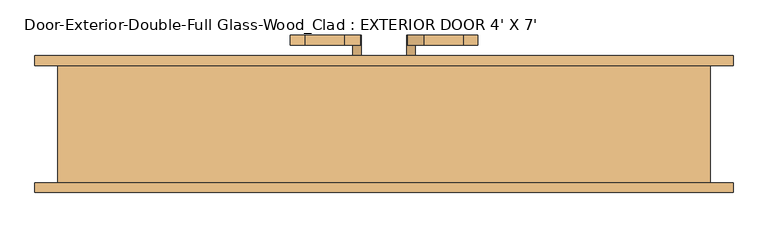
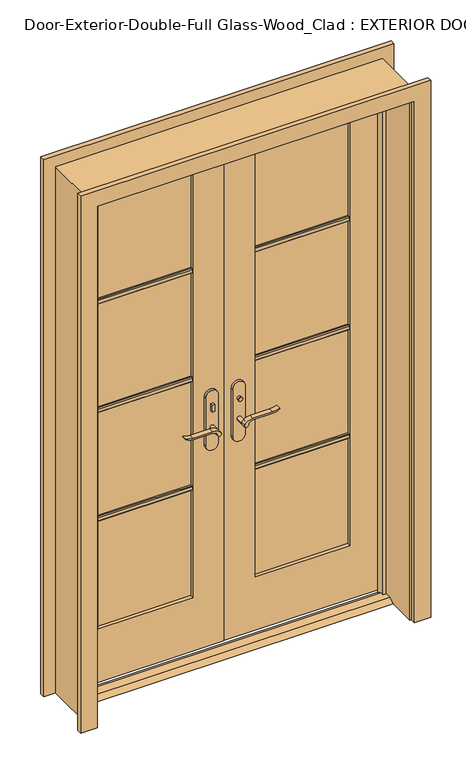
"""IFC4 building model written with IfcOpenShell, lengths in millimetres: door geometry, Door-Exterior-Double-Full Glass-Wood_Clad : EXTERIOR DOOR 4' X 7'."""

from ifc_helpers import new_model, si_unit, point, frame, frame_2d, origin, place, context, project, spatial, polyline, circle_curve, trimmed, segment, composite_curve, outline, extrude, faceted_brep, source, transform, mapped, element, save


def door_exterior_double_full_glass_wood_clad_exterior_door_4_x_3788f36b(model_context):
    return source(origin(), model_context, "Body", "SolidModel", [
        extrude(outline(polyline([(19.05, 12.7), (53.975, 12.7), (79.375, 0.0), (-6.35, 0.0), (19.05, 12.7)])), frame((-609.6, 0.0, 0.0), z_axis=(1.0, 0.0, 0.0), x_axis=(0.0, 1.0, 0.0)), (0.0, 0.0, 1.0), 1219.2),
        extrude(outline(polyline([(-47.4019111, 56.2), (-57.4019111, 56.2), (-57.4019111, 66.2), (-47.4019111, 66.2), (-47.4019111, 56.2)])), frame((0.0, 0.0, 981.9), z_axis=(0.0, 0.0, 1.0), x_axis=(1.0, 0.0, 0.0)), (0.0, 0.0, 1.0), 30.0),
        extrude(outline(composite_curve([segment(trimmed(circle_curve(frame_2d((996.9, -52.4019111)), 8.0), [point((996.9, -60.4019111))], [point((996.9, -44.4019111))], False, "CARTESIAN"), True, "CONTINUOUS"), segment(trimmed(circle_curve(frame_2d((996.9, -52.4019111)), 8.0), [point((996.9, -44.4019111))], [point((996.9, -60.4019111))], False, "CARTESIAN"), True, "CONTINUOUS")], self_intersect=False)), frame((0.0, 121.125, 0.0), z_axis=(0.0, 1.0, 0.0), x_axis=(0.0, 0.0, 1.0)), (0.0, 0.0, 1.0), 10.0),
        extrude(outline(composite_curve([segment(trimmed(circle_curve(frame_2d((897.1555521, -76.0694241)), 37.2832219), [point((919.0523287, -45.8937749))], [point((934.4, -77.7693445))], False, "CARTESIAN"), True, "CONTINUOUS"), segment(polyline([(934.4, -77.7693445), (934.4, -154.045502)]), True, "CONTINUOUS"), segment(trimmed(circle_curve(frame_2d((1017.6850638, -153.9791202)), 83.2850902), [point((934.4, -154.045502))], [point((939.4, -182.4019111))], True, "CARTESIAN"), True, "CONTINUOUS"), segment(polyline([(939.4, -182.4019111), (936.6135558, -182.4019111)]), True, "CONTINUOUS"), segment(trimmed(circle_curve(frame_2d((986.6709207, -150.4622499)), 59.3791355), [point((936.6135558, -182.4019111))], [point((927.4, -154.045502))], False, "CARTESIAN"), True, "CONTINUOUS"), segment(polyline([(927.4, -154.045502), (927.4, -77.7881013)]), True, "CONTINUOUS"), segment(trimmed(circle_curve(frame_2d((909.2738613, -77.7881013)), 18.1261387), [point((927.4, -77.7881013))], [point((914.4, -60.4019111))], True, "CARTESIAN"), True, "CONTINUOUS"), segment(trimmed(circle_curve(frame_2d((914.4, -52.4019111)), 8.0), [point((914.4, -60.4019111))], [point((919.0523287, -45.8937749))], False, "CARTESIAN"), True, "CONTINUOUS")], self_intersect=False)), frame((0.0, 16.2, 0.0), z_axis=(0.0, 1.0, 0.0), x_axis=(0.0, 0.0, 1.0)), (0.0, 0.0, 1.0), 20.0),
        extrude(outline(composite_curve([segment(trimmed(circle_curve(frame_2d((914.4, -52.4019111)), 8.0), [point((914.3999903, -60.4019111))], [point((919.0523287, -45.8937749))], False, "CARTESIAN"), True, "CONTINUOUS"), segment(trimmed(circle_curve(frame_2d((897.1555521, -76.0694241)), 37.2832219), [point((919.0523287, -45.8937749))], [point((934.4, -77.7693445))], False, "CARTESIAN"), True, "CONTINUOUS"), segment(polyline([(934.4, -77.7693445), (934.4, -154.045502)]), True, "CONTINUOUS"), segment(trimmed(circle_curve(frame_2d((1017.6850638, -153.9791202)), 83.2850902), [point((934.4, -154.045502))], [point((939.4, -182.4019111))], True, "CARTESIAN"), True, "CONTINUOUS"), segment(polyline([(939.4, -182.4019111), (936.6135558, -182.4019111)]), True, "CONTINUOUS"), segment(trimmed(circle_curve(frame_2d((986.6709207, -150.4622499)), 59.3791355), [point((936.6135558, -182.4019111))], [point((927.4, -154.045502))], False, "CARTESIAN"), True, "CONTINUOUS"), segment(polyline([(927.4, -154.045502), (927.4, -77.788099)]), True, "CONTINUOUS"), segment(trimmed(circle_curve(frame_2d((909.2738682, -77.788099)), 18.1261318), [point((927.4, -77.788099))], [point((914.3999903, -60.4019111))], True, "CARTESIAN"), True, "CONTINUOUS")], self_intersect=False)), frame((0.0, 151.125, 0.0), z_axis=(0.0, 1.0, 0.0), x_axis=(0.0, 0.0, 1.0)), (0.0, 0.0, 1.0), 20.0),
        extrude(outline(composite_curve([segment(trimmed(circle_curve(frame_2d((914.4, -52.4019111)), 8.0), [point((914.4, -60.4019111))], [point((914.4, -44.4019111))], False, "CARTESIAN"), True, "CONTINUOUS"), segment(trimmed(circle_curve(frame_2d((914.4, -52.4019111)), 8.0), [point((914.4, -44.4019111))], [point((914.4, -60.4019111))], False, "CARTESIAN"), True, "CONTINUOUS")], self_intersect=False)), frame((0.0, 36.2, 0.0), z_axis=(0.0, 1.0, 0.0), x_axis=(0.0, 0.0, 1.0)), (0.0, 0.0, 1.0), 30.0),
        extrude(outline(composite_curve([segment(trimmed(circle_curve(frame_2d((914.4, -52.4019111)), 8.0), [point((914.4, -60.4019111))], [point((914.4, -44.4019111))], False, "CARTESIAN"), True, "CONTINUOUS"), segment(trimmed(circle_curve(frame_2d((914.4, -52.4019111)), 8.0), [point((914.4, -44.4019111))], [point((914.4, -60.4019111))], False, "CARTESIAN"), True, "CONTINUOUS")], self_intersect=False)), frame((0.0, 121.125, 0.0), z_axis=(0.0, 1.0, 0.0), x_axis=(0.0, 0.0, 1.0)), (0.0, 0.0, 1.0), 30.0),
        extrude(outline(composite_curve([segment(polyline([(844.4, -27.4019111), (1039.4, -27.4019111)]), True, "CONTINUOUS"), segment(trimmed(circle_curve(frame_2d((1039.4, -52.4019111)), 25.0), [point((1039.4, -27.4019111))], [point((1039.4, -77.4019111))], False, "CARTESIAN"), True, "CONTINUOUS"), segment(polyline([(1039.4, -77.4019111), (844.4, -77.4019111)]), True, "CONTINUOUS"), segment(trimmed(circle_curve(frame_2d((844.4, -52.4019111)), 25.0), [point((844.4, -77.4019111))], [point((844.4, -27.4019111))], False, "CARTESIAN"), True, "CONTINUOUS")], self_intersect=False)), frame((0.0, 66.2, 0.0), z_axis=(0.0, 1.0, 0.0), x_axis=(0.0, 0.0, 1.0)), (0.0, 0.0, 1.0), 10.0),
        extrude(outline(composite_curve([segment(polyline([(844.4, -27.4019111), (1039.4, -27.4019111)]), True, "CONTINUOUS"), segment(trimmed(circle_curve(frame_2d((1039.4, -52.4019111)), 25.0), [point((1039.4, -27.4019111))], [point((1039.4, -77.4019111))], False, "CARTESIAN"), True, "CONTINUOUS"), segment(polyline([(1039.4, -77.4019111), (844.4, -77.4019111)]), True, "CONTINUOUS"), segment(trimmed(circle_curve(frame_2d((844.4, -52.4019111)), 25.0), [point((844.4, -77.4019111))], [point((844.4, -27.4019111))], False, "CARTESIAN"), True, "CONTINUOUS")], self_intersect=False)), frame((0.0, 111.125, 0.0), z_axis=(0.0, 1.0, 0.0), x_axis=(0.0, 0.0, 1.0)), (0.0, 0.0, 1.0), 10.0),
        extrude(outline(polyline([(47.3875, 131.125), (57.3875, 131.125), (57.3875, 121.125), (47.3875, 121.125), (47.3875, 131.125)])), frame((0.0, 0.0, 981.9), z_axis=(0.0, 0.0, 1.0), x_axis=(1.0, 0.0, 0.0)), (0.0, 0.0, 1.0), 30.0),
        extrude(outline(composite_curve([segment(trimmed(circle_curve(frame_2d((996.9, 52.3875)), 8.0), [point((996.9, 60.3875))], [point((996.9, 44.3875))], False, "CARTESIAN"), True, "CONTINUOUS"), segment(trimmed(circle_curve(frame_2d((996.9, 52.3875)), 8.0), [point((996.9, 44.3875))], [point((996.9, 60.3875))], False, "CARTESIAN"), True, "CONTINUOUS")], self_intersect=False)), frame((0.0, 56.2, 0.0), z_axis=(0.0, 1.0, 0.0), x_axis=(0.0, 0.0, 1.0)), (0.0, 0.0, 1.0), 10.0),
        extrude(outline(composite_curve([segment(trimmed(circle_curve(frame_2d((914.4, 52.3875)), 8.0), [point((919.0523287, 45.8793637))], [point((914.4, 60.3875))], False, "CARTESIAN"), True, "CONTINUOUS"), segment(trimmed(circle_curve(frame_2d((909.2738613, 77.7736901)), 18.1261387), [point((914.4, 60.3875))], [point((927.4, 77.7736901))], True, "CARTESIAN"), True, "CONTINUOUS"), segment(polyline([(927.4, 77.7736901), (927.4, 154.0310909)]), True, "CONTINUOUS"), segment(trimmed(circle_curve(frame_2d((986.6709207, 150.4478388)), 59.3791355), [point((927.4, 154.0310909))], [point((936.6135558, 182.3875))], False, "CARTESIAN"), True, "CONTINUOUS"), segment(polyline([(936.6135558, 182.3875), (939.4, 182.3875)]), True, "CONTINUOUS"), segment(trimmed(circle_curve(frame_2d((1017.6850638, 153.9647091)), 83.2850902), [point((939.4, 182.3875))], [point((934.4, 154.0310909))], True, "CARTESIAN"), True, "CONTINUOUS"), segment(polyline([(934.4, 154.0310909), (934.4, 77.7549333)]), True, "CONTINUOUS"), segment(trimmed(circle_curve(frame_2d((897.1555521, 76.0550129)), 37.2832219), [point((934.4, 77.7549333))], [point((919.0523287, 45.8793637))], False, "CARTESIAN"), True, "CONTINUOUS")], self_intersect=False)), frame((0.0, 151.125, 0.0), z_axis=(0.0, 1.0, 0.0), x_axis=(0.0, 0.0, 1.0)), (0.0, 0.0, 1.0), 20.0),
        extrude(outline(composite_curve([segment(trimmed(circle_curve(frame_2d((909.2738682, 77.7736878)), 18.1261318), [point((914.3999903, 60.3875))], [point((927.4, 77.7736878))], True, "CARTESIAN"), True, "CONTINUOUS"), segment(polyline([(927.4, 77.7736878), (927.4, 154.0310909)]), True, "CONTINUOUS"), segment(trimmed(circle_curve(frame_2d((986.6709207, 150.4478388)), 59.3791355), [point((927.4, 154.0310909))], [point((936.6135558, 182.3875))], False, "CARTESIAN"), True, "CONTINUOUS"), segment(polyline([(936.6135558, 182.3875), (939.4, 182.3875)]), True, "CONTINUOUS"), segment(trimmed(circle_curve(frame_2d((1017.6850638, 153.9647091)), 83.2850902), [point((939.4, 182.3875))], [point((934.4, 154.0310909))], True, "CARTESIAN"), True, "CONTINUOUS"), segment(polyline([(934.4, 154.0310909), (934.4, 77.7549333)]), True, "CONTINUOUS"), segment(trimmed(circle_curve(frame_2d((897.1555521, 76.0550129)), 37.2832219), [point((934.4, 77.7549333))], [point((919.0523287, 45.8793637))], False, "CARTESIAN"), True, "CONTINUOUS"), segment(trimmed(circle_curve(frame_2d((914.4, 52.3875)), 8.0), [point((919.0523287, 45.8793637))], [point((914.3999903, 60.3875))], False, "CARTESIAN"), True, "CONTINUOUS")], self_intersect=False)), frame((0.0, 16.2, 0.0), z_axis=(0.0, 1.0, 0.0), x_axis=(0.0, 0.0, 1.0)), (0.0, 0.0, 1.0), 20.0),
        extrude(outline(composite_curve([segment(trimmed(circle_curve(frame_2d((914.4, 52.3875)), 8.0), [point((914.4, 60.3875))], [point((914.4, 44.3875))], False, "CARTESIAN"), True, "CONTINUOUS"), segment(trimmed(circle_curve(frame_2d((914.4, 52.3875)), 8.0), [point((914.4, 44.3875))], [point((914.4, 60.3875))], False, "CARTESIAN"), True, "CONTINUOUS")], self_intersect=False)), frame((0.0, 121.125, 0.0), z_axis=(0.0, 1.0, 0.0), x_axis=(0.0, 0.0, 1.0)), (0.0, 0.0, 1.0), 30.0),
        extrude(outline(composite_curve([segment(trimmed(circle_curve(frame_2d((914.4, 52.3875)), 8.0), [point((914.4, 60.3875))], [point((914.4, 44.3875))], False, "CARTESIAN"), True, "CONTINUOUS"), segment(trimmed(circle_curve(frame_2d((914.4, 52.3875)), 8.0), [point((914.4, 44.3875))], [point((914.4, 60.3875))], False, "CARTESIAN"), True, "CONTINUOUS")], self_intersect=False)), frame((0.0, 36.2, 0.0), z_axis=(0.0, 1.0, 0.0), x_axis=(0.0, 0.0, 1.0)), (0.0, 0.0, 1.0), 30.0),
        extrude(outline(composite_curve([segment(trimmed(circle_curve(frame_2d((844.4, 52.3875)), 25.0), [point((844.4, 27.3875))], [point((844.4, 77.3875))], False, "CARTESIAN"), True, "CONTINUOUS"), segment(polyline([(844.4, 77.3875), (1039.4, 77.3875)]), True, "CONTINUOUS"), segment(trimmed(circle_curve(frame_2d((1039.4, 52.3875)), 25.0), [point((1039.4, 77.3875))], [point((1039.4, 27.3875))], False, "CARTESIAN"), True, "CONTINUOUS"), segment(polyline([(1039.4, 27.3875), (844.4, 27.3875)]), True, "CONTINUOUS")], self_intersect=False)), frame((0.0, 111.125, 0.0), z_axis=(0.0, 1.0, 0.0), x_axis=(0.0, 0.0, 1.0)), (0.0, 0.0, 1.0), 10.0),
        extrude(outline(composite_curve([segment(trimmed(circle_curve(frame_2d((844.4, 52.3875)), 25.0), [point((844.4, 27.3875))], [point((844.4, 77.3875))], False, "CARTESIAN"), True, "CONTINUOUS"), segment(polyline([(844.4, 77.3875), (1039.4, 77.3875)]), True, "CONTINUOUS"), segment(trimmed(circle_curve(frame_2d((1039.4, 52.3875)), 25.0), [point((1039.4, 77.3875))], [point((1039.4, 27.3875))], False, "CARTESIAN"), True, "CONTINUOUS"), segment(polyline([(1039.4, 27.3875), (844.4, 27.3875)]), True, "CONTINUOUS")], self_intersect=False)), frame((0.0, 66.2, 0.0), z_axis=(0.0, 1.0, 0.0), x_axis=(0.0, 0.0, 1.0)), (0.0, 0.0, 1.0), 10.0),
        extrude(outline(polyline([(90.17, 1578.371875), (90.17, 1559.321875), (83.82, 1559.321875), (80.645, 1562.496875), (80.645, 1575.196875), (83.82, 1578.371875), (90.17, 1578.371875)])), frame((120.65, 0.0, 0.0), z_axis=(1.0, 0.0, 0.0), x_axis=(0.0, 1.0, 0.0)), (0.0, 0.0, 1.0), 368.3),
        extrude(outline(polyline([(90.17, 1132.68125), (90.17, 1113.63125), (83.82, 1113.63125), (80.645, 1116.80625), (80.645, 1129.50625), (83.82, 1132.68125), (90.17, 1132.68125)])), frame((120.65, 0.0, 0.0), z_axis=(1.0, 0.0, 0.0), x_axis=(0.0, 1.0, 0.0)), (0.0, 0.0, 1.0), 368.3),
        extrude(outline(polyline([(90.17, 686.990625), (90.17, 667.940625), (83.82, 667.940625), (80.645, 671.115625), (80.645, 683.815625), (83.82, 686.990625), (90.17, 686.990625)])), frame((120.65, 0.0, 0.0), z_axis=(1.0, 0.0, 0.0), x_axis=(0.0, 1.0, 0.0)), (0.0, 0.0, 1.0), 368.3),
        extrude(outline(polyline([(97.155, 1578.371875), (103.505, 1578.371875), (106.68, 1575.196875), (106.68, 1562.496875), (103.505, 1559.321875), (97.155, 1559.321875), (97.155, 1578.371875)])), frame((-488.95, 0.0, 0.0), z_axis=(1.0, 0.0, 0.0), x_axis=(0.0, 1.0, 0.0)), (0.0, 0.0, 1.0), 368.3),
        extrude(outline(polyline([(97.155, 1132.68125), (103.505, 1132.68125), (106.68, 1129.50625), (106.68, 1116.80625), (103.505, 1113.63125), (97.155, 1113.63125), (97.155, 1132.68125)])), frame((-488.95, 0.0, 0.0), z_axis=(1.0, 0.0, 0.0), x_axis=(0.0, 1.0, 0.0)), (0.0, 0.0, 1.0), 368.3),
        extrude(outline(polyline([(97.155, 686.990625), (103.505, 686.990625), (106.68, 683.815625), (106.68, 671.115625), (103.505, 667.940625), (97.155, 667.940625), (97.155, 686.990625)])), frame((-488.95, 0.0, 0.0), z_axis=(1.0, 0.0, 0.0), x_axis=(0.0, 1.0, 0.0)), (0.0, 0.0, 1.0), 368.3),
        extrude(outline(polyline([(97.155, 1578.371875), (103.505, 1578.371875), (106.68, 1575.196875), (106.68, 1562.496875), (103.505, 1559.321875), (97.155, 1559.321875), (97.155, 1578.371875)])), frame((120.65, 0.0, 0.0), z_axis=(1.0, 0.0, 0.0), x_axis=(0.0, 1.0, 0.0)), (0.0, 0.0, 1.0), 368.3),
        extrude(outline(polyline([(97.155, 1132.68125), (103.505, 1132.68125), (106.68, 1129.50625), (106.68, 1116.80625), (103.505, 1113.63125), (97.155, 1113.63125), (97.155, 1132.68125)])), frame((120.65, 0.0, 0.0), z_axis=(1.0, 0.0, 0.0), x_axis=(0.0, 1.0, 0.0)), (0.0, 0.0, 1.0), 368.3),
        extrude(outline(polyline([(97.155, 686.990625), (103.505, 686.990625), (106.68, 683.815625), (106.68, 671.115625), (103.505, 667.940625), (97.155, 667.940625), (97.155, 686.990625)])), frame((120.65, 0.0, 0.0), z_axis=(1.0, 0.0, 0.0), x_axis=(0.0, 1.0, 0.0)), (0.0, 0.0, 1.0), 368.3),
        extrude(outline(polyline([(90.17, 1578.371875), (90.17, 1559.321875), (83.82, 1559.321875), (80.645, 1562.496875), (80.645, 1575.196875), (83.82, 1578.371875), (90.17, 1578.371875)])), frame((-488.95, 0.0, 0.0), z_axis=(1.0, 0.0, 0.0), x_axis=(0.0, 1.0, 0.0)), (0.0, 0.0, 1.0), 368.3),
        extrude(outline(polyline([(90.17, 1132.68125), (90.17, 1113.63125), (83.82, 1113.63125), (80.645, 1116.80625), (80.645, 1129.50625), (83.82, 1132.68125), (90.17, 1132.68125)])), frame((-488.95, 0.0, 0.0), z_axis=(1.0, 0.0, 0.0), x_axis=(0.0, 1.0, 0.0)), (0.0, 0.0, 1.0), 368.3),
        extrude(outline(polyline([(90.17, 686.990625), (90.17, 667.940625), (83.82, 667.940625), (80.645, 671.115625), (80.645, 683.815625), (83.82, 686.990625), (90.17, 686.990625)])), frame((-488.95, 0.0, 0.0), z_axis=(1.0, 0.0, 0.0), x_axis=(0.0, 1.0, 0.0)), (0.0, 0.0, 1.0), 368.3),
        extrude(outline(polyline([(0.0, 615.95), (0.0, 679.45), (2203.45, 679.45), (2203.45, -679.45), (0.0, -679.45), (0.0, -615.95), (2139.95, -615.95), (2139.95, 615.95), (0.0, 615.95)])), frame((0.0, -136.525, 0.0), z_axis=(0.0, 1.0, 0.0), x_axis=(0.0, 0.0, 1.0)), (0.0, 0.0, 1.0), 19.05),
        extrude(outline(polyline([(0.0, 615.95), (0.0, 679.45), (2203.45, 679.45), (2203.45, -679.45), (0.0, -679.45), (0.0, -615.95), (2139.95, -615.95), (2139.95, 615.95), (0.0, 615.95)])), frame((0.0, 111.125, 0.0), z_axis=(0.0, 1.0, 0.0), x_axis=(0.0, 0.0, 1.0)), (0.0, 0.0, 1.0), 19.05),
        faceted_brep([(635.0, 111.125, 0.0), (635.0, -117.475, 0.0), (609.6, -117.475, 0.0), (609.6, 41.275, 0.0), (596.9, 41.275, 0.0), (596.9, 76.2, 0.0), (609.6, 76.2, 0.0), (609.6, 111.125, 0.0), (635.0, 111.125, 2159.0), (635.0, -117.475, 2159.0), (-635.0, -117.475, 2159.0), (-635.0, -117.475, 0.0), (-609.6, -117.475, 0.0), (-609.6, -117.475, 2133.6), (609.6, -117.475, 2133.6), (609.6, 41.275, 2133.6), (-609.6, 41.275, 2133.6), (-609.6, 41.275, 0.0), (-596.9, 41.275, 0.0), (-596.9, 41.275, 2120.9), (596.9, 41.275, 2120.9), (596.9, 76.2, 2120.9), (1.5875, 76.2, 2120.9), (-1.6019111, 76.2, 2120.9), (-596.9, 76.2, 2120.9), (-596.9, 76.2, 0.0), (-609.6, 76.2, 0.0), (-609.6, 76.2, 2133.6), (-1.6019111, 76.2, 2133.6), (1.5875, 76.2, 2133.6), (609.6, 76.2, 2133.6), (609.6, 111.125, 2133.6), (1.5875, 111.125, 2133.6), (-1.6019111, 111.125, 2133.6), (-609.6, 111.125, 2133.6), (-609.6, 111.125, 0.0), (-635.0, 111.125, 0.0), (-635.0, 111.125, 2159.0)], [[[0, 1, 2, 3, 4, 5, 6, 7]], [[1, 0, 8, 9]], [[2, 1, 9, 10, 11, 12, 13, 14]], [[3, 2, 14, 15]], [[4, 3, 15, 16, 17, 18, 19, 20]], [[5, 4, 20, 21]], [[6, 5, 21, 22, 23, 24, 25, 26, 27, 28, 29, 30]], [[7, 6, 30, 31]], [[0, 7, 31, 32, 33, 34, 35, 36, 37, 8]], [[9, 8, 37, 10]], [[14, 13, 16, 15]], [[20, 19, 24, 23, 22, 21]], [[31, 30, 29, 28, 27, 34, 33, 32]], [[12, 11, 36, 35, 26, 25, 18, 17]], [[11, 10, 37, 36]], [[13, 12, 17, 16]], [[19, 18, 25, 24]], [[27, 26, 35, 34]]]),
        extrude(outline(polyline([(12.7, 609.6), (2133.6, 609.6), (2133.6, 1.5875), (12.7, 1.5875), (12.7, 609.6)]), holes=[polyline([(2014.5375, 120.65), (2014.5375, 488.95), (231.775, 488.95), (231.775, 120.65), (2014.5375, 120.65)])]), frame((0.0, 76.2, 0.0), z_axis=(0.0, 1.0, 0.0), x_axis=(0.0, 0.0, 1.0)), (0.0, 0.0, 1.0), 34.925),
        extrude(outline(polyline([(2133.6, -609.6), (12.7, -609.6), (12.7, -1.6019111), (2133.6, -1.6019111), (2133.6, -609.6)]), holes=[polyline([(231.775, -488.95), (2014.5375, -488.95), (2014.5375, -120.65), (231.775, -120.65), (231.775, -488.95)])]), frame((0.0, 76.2, 0.0), z_axis=(0.0, 1.0, 0.0), x_axis=(0.0, 0.0, 1.0)), (0.0, 0.0, 1.0), 34.925),
        extrude(outline(polyline([(488.95, 90.17), (120.65, 90.17), (120.65, 97.155), (488.95, 97.155), (488.95, 90.17)])), frame((0.0, 0.0, 231.775), z_axis=(0.0, 0.0, 1.0), x_axis=(1.0, 0.0, 0.0)), (0.0, 0.0, 1.0), 1782.7625),
        extrude(outline(polyline([(-120.65, 90.17), (-488.95, 90.17), (-488.95, 97.155), (-120.65, 97.155), (-120.65, 90.17)])), frame((0.0, 0.0, 231.775), z_axis=(0.0, 0.0, 1.0), x_axis=(1.0, 0.0, 0.0)), (0.0, 0.0, 1.0), 1782.7625),
    ])


if __name__ == "__main__":
    model = new_model("IFC4")
    model_context = context("Model", 3, world=origin())
    ifc_project = project(units=[si_unit("LENGTHUNIT", "METRE", prefix="MILLI")], contexts=[model_context])
    site = spatial("IfcSite", under=ifc_project)
    building = spatial("IfcBuilding", under=site)
    placement = place(None, origin())
    door_exterior_double_full_glass_wood_clad_exterior_door_4_x_shape = door_exterior_double_full_glass_wood_clad_exterior_door_4_x_3788f36b(model_context)
    element("IfcDoor", 1, ObjectType="Door-Exterior-Double-Full Glass-Wood_Clad : EXTERIOR DOOR 4' X 7'", at=placement, inside=building, context=model_context, shape_type="MappedRepresentation", body=[
        mapped(door_exterior_double_full_glass_wood_clad_exterior_door_4_x_shape, transform((0.0, 0.0, 0.0), x_axis=(1.0, 0.0, 0.0), y_axis=(0.0, 1.0, 0.0), z_axis=(0.0, 0.0, 1.0))),
    ])
    save(model, "model.ifc")

# Revit data of these elements
# Type "Door-Exterior-Double-Full Glass-Wood_Clad : EXTERIOR DOOR 4' X 7'"
#   Type Mark = "9"
#   Assembly Code = "B2030100"
#   Analytic Construction = "French door, wood frame with double glass"
#   Top Rail = 0' - 4 11/16"
#   Threshold Offset [instance default] = 0' - 0 1/2"
#   Thickness = 0' - 1 3/8"
#   Thermal Resistance (R) = 1.9158 (h·ft²·°F)/BTU
#   Swing Angle [instance default] = 90.00°
#   Stiles = 0' - 4 3/4"
#   Rough Width = 4' - 2"
#   Rough Height = 7' - 1"
#   Panel Width = 2' - 0"
#   Door Offset [instance default] = 0' - 0"
#   Height = 7' - 0"
#   Width = 4' - 0"
#   Heat Transfer Coefficient (U) = 0.5220 BTU/(h·ft²·°F)
#   Bottom Rail = 0' - 9 1/8"
#   Exterior Trim [instance default] = yes
#   Threshold [instance default] = yes
#   Show Grill [instance default] = yes
#   Function = 1
#   Trim Material = Cherry
#   Threshold Material = Cherry
#   Panel Material = Cherry
#   Glazing = Glass
#   Frame Material = Cherry
#   Door Handle Material = Aluminum
#   Visual Light Transmittance = 0
#   Solar Heat Gain Coefficient = 0
#   Wall Closure = (empty or 0)
#   Construction Type = (empty or 0)
# Element 1 (IfcDoor, "Door-Exterior-Double-Full Glass-Wood_Clad : EXTERIOR DOOR 4' X 7'")
#   Materials on its faces: "Cherry", "Aluminum", "Glass"
# Materials
#   "Cherry": class "Wood", colour RGB 226 177 128, transparency 0, Description = "Prunus Serotina", Cost = 0
#   "Glass": class "Glass", colour RGB 0 128 192, transparency 0.75, Description = "Soda Lime Glass", Cost = 0
#   "Aluminum": class "Metal", colour RGB 247 247 247, transparency 0, Description = "Aluminum 6061", Cost = 0
